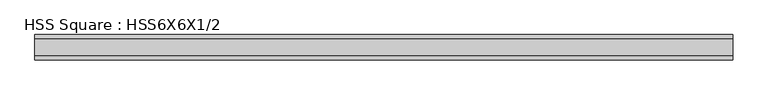
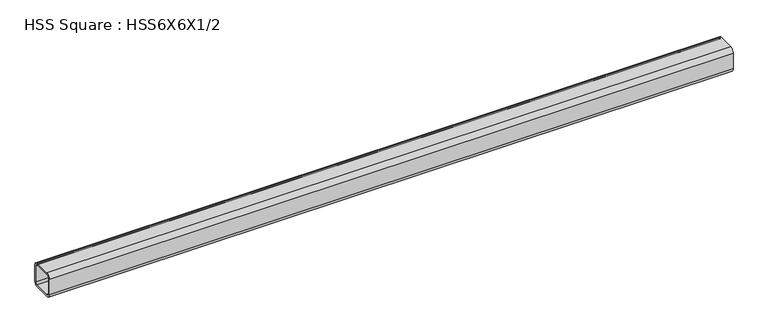
"""IFC4 building model written with IfcOpenShell, lengths in millimetres: member geometry, HSS Square : HSS6X6X1/2."""

from ifc_helpers import new_model, si_unit, point, frame, frame_2d, origin, place, context, project, spatial, polyline, circle_curve, trimmed, segment, composite_curve, outline, extrude, source, transform, mapped, element, save


def hss_square_hss6x6x1_2_10b7330d(model_context):
    return source(origin(), model_context, "Body", "SweptSolid", [
        extrude(outline(composite_curve([segment(trimmed(circle_curve(frame_2d((-50.8, 50.8)), 25.4), [point((-76.2, 50.8))], [point((-50.8, 76.2))], False, "CARTESIAN"), True, "CONTINUOUS"), segment(polyline([(-50.8, 76.2), (50.8, 76.2)]), True, "CONTINUOUS"), segment(trimmed(circle_curve(frame_2d((50.8, 50.8)), 25.4), [point((50.8, 76.2))], [point((76.2, 50.8))], False, "CARTESIAN"), True, "CONTINUOUS"), segment(polyline([(76.2, 50.8), (76.2, -50.8)]), True, "CONTINUOUS"), segment(trimmed(circle_curve(frame_2d((50.8, -50.8)), 25.4), [point((76.2, -50.8))], [point((50.8, -76.2))], False, "CARTESIAN"), True, "CONTINUOUS"), segment(polyline([(50.8, -76.2), (-50.8, -76.2)]), True, "CONTINUOUS"), segment(trimmed(circle_curve(frame_2d((-50.8, -50.8)), 25.4), [point((-50.8, -76.2))], [point((-76.2, -50.8))], False, "CARTESIAN"), True, "CONTINUOUS"), segment(polyline([(-76.2, -50.8), (-76.2, 50.8)]), True, "CONTINUOUS")], self_intersect=False), holes=[composite_curve([segment(polyline([(50.8, 63.5), (-50.8, 63.5)]), True, "CONTINUOUS"), segment(trimmed(circle_curve(frame_2d((-50.8, 50.8)), 12.7), [point((-50.8, 63.5))], [point((-63.5, 50.8))], True, "CARTESIAN"), True, "CONTINUOUS"), segment(polyline([(-63.5, 50.8), (-63.5, -50.8)]), True, "CONTINUOUS"), segment(trimmed(circle_curve(frame_2d((-50.8, -50.8)), 12.7), [point((-63.5, -50.8))], [point((-50.8, -63.5))], True, "CARTESIAN"), True, "CONTINUOUS"), segment(polyline([(-50.8, -63.5), (50.8, -63.5)]), True, "CONTINUOUS"), segment(trimmed(circle_curve(frame_2d((50.8, -50.8)), 12.7), [point((50.8, -63.5))], [point((63.5, -50.8))], True, "CARTESIAN"), True, "CONTINUOUS"), segment(polyline([(63.5, -50.8), (63.5, 50.8)]), True, "CONTINUOUS"), segment(trimmed(circle_curve(frame_2d((50.8, 50.8)), 12.7), [point((63.5, 50.8))], [point((50.8, 63.5))], True, "CARTESIAN"), True, "CONTINUOUS")], self_intersect=False)]), frame((-2237.2689682, 0.0, 0.0), z_axis=(1.0, 0.0, 0.0), x_axis=(0.0, 1.0, 0.0)), (0.0, 0.0, 1.0), 4174.6532362),
    ])


if __name__ == "__main__":
    model = new_model("IFC4")
    model_context = context("Model", 3, world=origin())
    ifc_project = project(units=[si_unit("LENGTHUNIT", "METRE", prefix="MILLI")], contexts=[model_context])
    site = spatial("IfcSite", under=ifc_project)
    building = spatial("IfcBuilding", under=site)
    placement = place(None, origin())
    hss_square_hss6x6x1_2_shape = hss_square_hss6x6x1_2_10b7330d(model_context)
    element("IfcMember", 1, ObjectType="HSS Square : HSS6X6X1/2", at=placement, inside=building, context=model_context, shape_type="MappedRepresentation", body=[
        mapped(hss_square_hss6x6x1_2_shape, transform((0.0, 0.0, 0.0), x_axis=(1.0, 0.0, 0.0), y_axis=(0.0, 1.0, 0.0), z_axis=(0.0, 0.0, 1.0))),
    ])
    save(model, "model.ifc")

# Revit data of these elements
# Type "HSS Square : HSS6X6X1/2"
#   Section Name Key = "HSS 6X6X1/2"
#   Assembly Code = "B10"
#   Width = 6.000"
#   Wall Nominal Thickness = 0.500"
#   Wall Design Thickness = 0.465"
#   Torsional Moment of Inertia = 81.10 in⁴
#   Torsional Modulus = 28.10 in³
#   Section Area = 9.74 in²
#   Plastic Modulus weak axis = 19.80 in³
#   Plastic Modulus strong axis = 19.80 in³
#   Outer Fillet = 1.000"
#   Nominal Weight = 35.24 lbf/ft
#   Moment of Inertia weak axis = 48.30 in⁴
#   Moment of Inertia strong axis = 48.30 in⁴
#   Inner Fillet = 0.500"
#   Height = 6.000"
#   Elastic Modulus weak axis = 16.10 in³
#   Elastic Modulus strong axis = 16.10 in³
#   Centroid Vertical = 3.000"
#   Centroid Horizontal = 3.000"
#   Length [instance default] = 5' - 0"
#   Structural Material [instance default] = Steel ASTM A500, Grade B, Rectangular and Square
#   Principal Axes Angle = 0
# Element 1 (IfcMember, "HSS Square : HSS6X6X1/2")
#   Structural Material = Steel ASTM A992
#   Materials on its faces: "Steel ASTM A992"
# Materials
#   "Steel ASTM A500, Grade B, Rectangular and Square": class "Metal", colour RGB 199 199 199, transparency 0, Description = "Carbon steel", Cost = 0
#   "Steel ASTM A992": class "Metal", colour RGB 199 199 199, transparency 0, Description = "Structural steel 50ksi", Cost = 0
